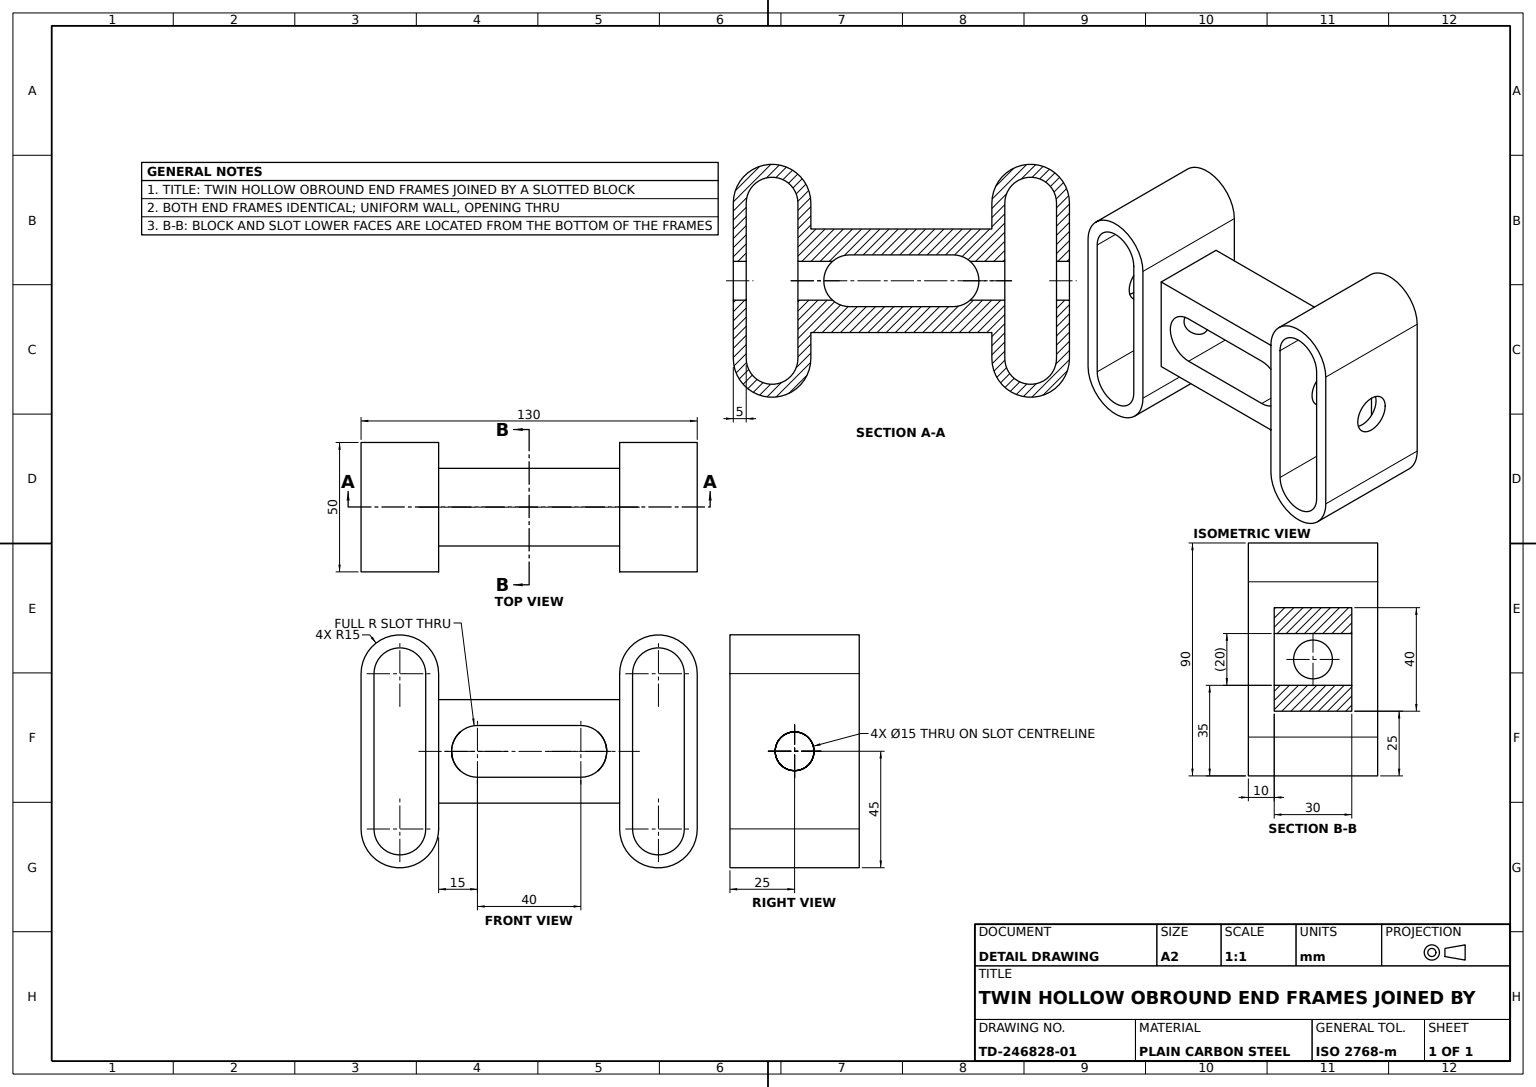
from build123d import *

# Parameters (mm, degrees)
CENTRE_BLOCK_PROFILE_W = 70
CENTRE_BLOCK_PROFILE_H = 40
CENTRE_BLOCK_DEPTH     = 30
END_LOOPS_DEPTH        = 25
CROSS_HOLE_PROFILE_R   = 7.5
CROSS_HOLE_15_DEPTH    = 95


with BuildPart() as part:
    # Centre Block Profile → Centre Block (new body)
    with BuildSketch(Plane.XY):
        Rectangle(CENTRE_BLOCK_PROFILE_W, CENTRE_BLOCK_PROFILE_H)
        with BuildLine():
            Line((20, -10), (-20, -10))
            ThreePointArc((-20, -10), (-30, 0), (-20, 10))
            Line((-20, 10), (20, 10))
            ThreePointArc((20, 10), (30, 0), (20, -10))
        make_face(mode=Mode.SUBTRACT)
    extrude(amount=CENTRE_BLOCK_DEPTH)

    # End Loops Profile → End Loops (add, symmetric)
    # profile 1 of 2: a face of its own
    with BuildSketch(Plane.XY.offset(15)):
        with BuildLine():
            Line((65, 30), (65, -30))
            ThreePointArc((65, -30), (50, -45), (35, -30))
            Line((35, -30), (35, 30))
            ThreePointArc((35, 30), (50, 45), (65, 30))
        make_face()
        with BuildLine():
            Line((60, 30), (60, -30))
            ThreePointArc((60, -30), (50, -40), (40, -30))
            Line((40, -30), (40, 30))
            ThreePointArc((40, 30), (50, 40), (60, 30))
        make_face(mode=Mode.SUBTRACT)
    # profile 2 of 2: a face of its own
    with BuildSketch(Plane.XY.offset(15)):
        with BuildLine():
            Line((-65, 30), (-65, -30))
            ThreePointArc((-65, -30), (-50, -45), (-35, -30))
            Line((-35, -30), (-35, 30))
            ThreePointArc((-35, 30), (-50, 45), (-65, 30))
        make_face()
        with BuildLine():
            Line((-40, 30), (-40, -30))
            ThreePointArc((-40, -30), (-50, -40), (-60, -30))
            Line((-60, -30), (-60, 30))
            ThreePointArc((-60, 30), (-50, 40), (-40, 30))
        make_face(mode=Mode.SUBTRACT)
    extrude(amount=END_LOOPS_DEPTH, both=True)

    # Cross Hole Profile → Cross Hole Ø15 (cut, symmetric)
    with BuildSketch(Plane(origin=(0, 0, 0), x_dir=(0, 0, -1), z_dir=(1, 0, 0))):
        with Locations(Location((-15, 0, 0), (0, 0, 270))):
            Circle(CROSS_HOLE_PROFILE_R)
    extrude(amount=CROSS_HOLE_15_DEPTH, both=True, mode=Mode.SUBTRACT)


solid = part.part
